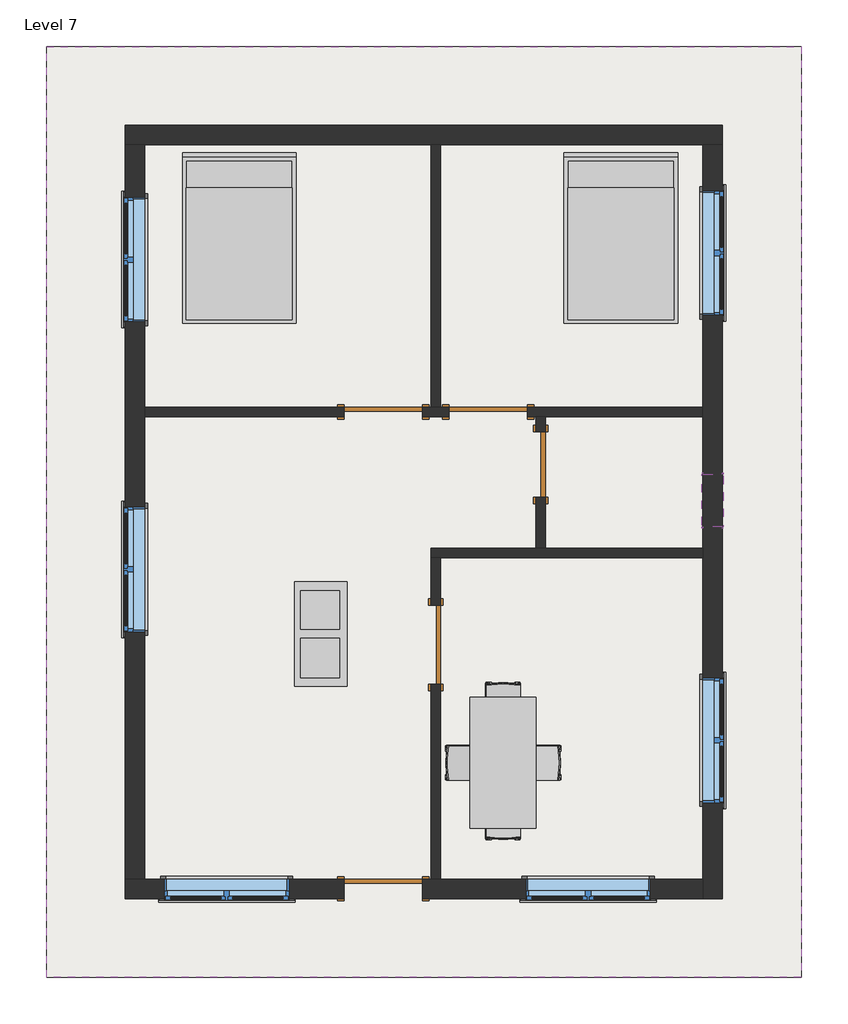
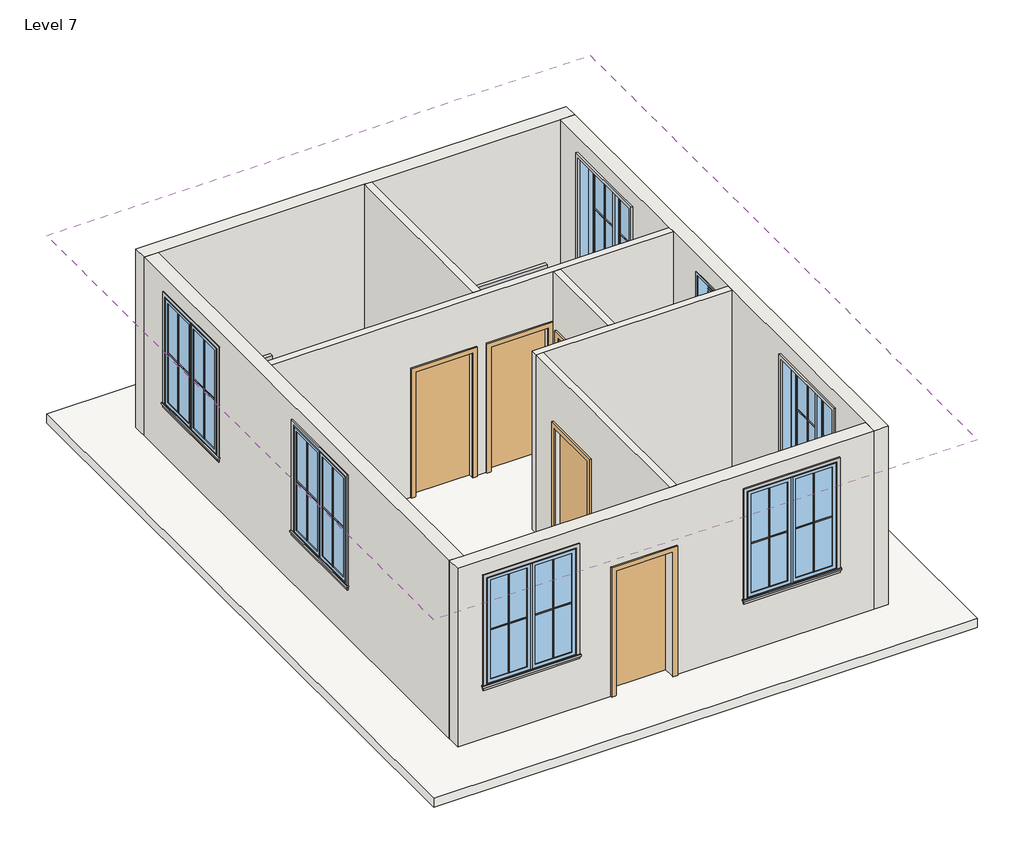
# One storey, incomplete: 25 proxies, 9 walls, 7 windows, 5 doors, 3 furniture elements, 2 roofs.
"""IFC4 building model written with IfcOpenShell, lengths in millimetres."""

from ifc_helpers import new_model, si_unit, frame, origin, place, context, project, spatial, polyline, outline, extrude, faceted_brep, transform, mapped, element, save
from components import muntin_pattern_2x2_muntin_pattern_2x2_bff912c5, muntin_pattern_2x2_muntin_pattern_2x2_c2194282, trim_window_exterior_flat_with_sill_e04b3088, trim_window_interior_flat_picture_frame_2a7685fe, coffee_table_with_brass_mullions_11320_coffee_table_with_5962bef7, door_305aa2a5, door_e5f9f3c4, door_0ca8825f, door_f2b275c1, bed_17739_bed_17739_15c61121, dining_table_w_chairs_11374_0cdfc61b, window_9ac97e1a, window_f2d8fef0

model = new_model("IFC4")

# Units and contexts
model_context = context("Model", 3, world=origin())
ifc_project = project(units=[si_unit("LENGTHUNIT", "METRE", prefix="MILLI")], contexts=[model_context])

# Site, building, storey
site = spatial("IfcSite", under=ifc_project)
building = spatial("IfcBuilding", under=site)
storey = spatial("IfcBuildingStorey", under=building, Name="Level 7", Elevation=19050.0)

# Proxies
placement = place(None, origin())
muntin_pattern_2x2_muntin_pattern_2x2_shape = muntin_pattern_2x2_muntin_pattern_2x2_bff912c5(model_context)
element("IfcBuildingElementProxy", 1, Name="Muntin Pattern_2x2 : Muntin Pattern_2x2", ObjectType="Muntin Pattern_2x2 : Muntin Pattern_2x2", at=placement, inside=storey, context=model_context, shape_type="MappedRepresentation", body=[
    mapped(muntin_pattern_2x2_muntin_pattern_2x2_shape, transform((-4718.1437352, -1580.3188735, 20034.25), x_axis=(0.0, 1.0, 0.0), y_axis=(-1.0, 0.0, 0.0), z_axis=(0.0, 0.0, 1.0))),
])
element("IfcBuildingElementProxy", 2, Name="Muntin Pattern_2x2 : Muntin Pattern_2x2", ObjectType="Muntin Pattern_2x2 : Muntin Pattern_2x2", at=placement, inside=storey, context=model_context, shape_type="MappedRepresentation", body=[
    mapped(muntin_pattern_2x2_muntin_pattern_2x2_shape, transform((-3186.2062352, -5039.4813735, 20034.25), x_axis=(-1.0, 0.0, 0.0), y_axis=(0.0, -1.0, 0.0), z_axis=(0.0, 0.0, 1.0))),
])
element("IfcBuildingElementProxy", 3, Name="Muntin Pattern_2x2 : Muntin Pattern_2x2", ObjectType="Muntin Pattern_2x2 : Muntin Pattern_2x2", at=placement, inside=storey, context=model_context, shape_type="MappedRepresentation", body=[
    mapped(muntin_pattern_2x2_muntin_pattern_2x2_shape, transform((1017.4937648, -5039.4813735, 20034.25), x_axis=(-1.0, 0.0, 0.0), y_axis=(0.0, -1.0, 0.0), z_axis=(0.0, 0.0, 1.0))),
])
element("IfcBuildingElementProxy", 4, Name="Muntin Pattern_2x2 : Muntin Pattern_2x2", ObjectType="Muntin Pattern_2x2 : Muntin Pattern_2x2", at=placement, inside=storey, context=model_context, shape_type="MappedRepresentation", body=[
    mapped(muntin_pattern_2x2_muntin_pattern_2x2_shape, transform((2209.7062648, -2847.1438735, 20034.25), x_axis=(0.0, -1.0, 0.0), y_axis=(1.0, 0.0, 0.0), z_axis=(0.0, 0.0, 1.0))),
])
element("IfcBuildingElementProxy", 5, Name="Muntin Pattern_2x2 : Muntin Pattern_2x2", ObjectType="Muntin Pattern_2x2 : Muntin Pattern_2x2", at=placement, inside=storey, context=model_context, shape_type="MappedRepresentation", body=[
    mapped(muntin_pattern_2x2_muntin_pattern_2x2_shape, transform((2209.7062648, 2817.0561265, 20034.25), x_axis=(0.0, -1.0, 0.0), y_axis=(1.0, 0.0, 0.0), z_axis=(0.0, 0.0, 1.0))),
])
element("IfcBuildingElementProxy", 6, Name="Muntin Pattern_2x2 : Muntin Pattern_2x2", ObjectType="Muntin Pattern_2x2 : Muntin Pattern_2x2", at=placement, inside=storey, context=model_context, shape_type="MappedRepresentation", body=[
    mapped(muntin_pattern_2x2_muntin_pattern_2x2_shape, transform((-4718.1437352, 2020.1311265, 20034.25), x_axis=(0.0, 1.0, 0.0), y_axis=(-1.0, 0.0, 0.0), z_axis=(0.0, 0.0, 1.0))),
])
muntin_pattern_2x2_muntin_pattern_2x2_2_shape = muntin_pattern_2x2_muntin_pattern_2x2_c2194282(model_context)
element("IfcBuildingElementProxy", 7, Name="Muntin Pattern_2x2 : Muntin Pattern_2x2", ObjectType="Muntin Pattern_2x2 : Muntin Pattern_2x2", at=placement, inside=storey, context=model_context, shape_type="MappedRepresentation", body=[
    mapped(muntin_pattern_2x2_muntin_pattern_2x2_2_shape, transform((-4718.1437352, -859.5938735, 20034.25), x_axis=(0.0, -1.0, 0.0), y_axis=(1.0, 0.0, 0.0), z_axis=(0.0, 0.0, 1.0))),
])
element("IfcBuildingElementProxy", 8, Name="Muntin Pattern_2x2 : Muntin Pattern_2x2", ObjectType="Muntin Pattern_2x2 : Muntin Pattern_2x2", at=placement, inside=storey, context=model_context, shape_type="MappedRepresentation", body=[
    mapped(muntin_pattern_2x2_muntin_pattern_2x2_2_shape, transform((-3906.9312352, -5039.4813735, 20034.25), x_axis=(1.0, 0.0, 0.0), y_axis=(0.0, 1.0, 0.0), z_axis=(0.0, 0.0, 1.0))),
])
element("IfcBuildingElementProxy", 9, Name="Muntin Pattern_2x2 : Muntin Pattern_2x2", ObjectType="Muntin Pattern_2x2 : Muntin Pattern_2x2", at=placement, inside=storey, context=model_context, shape_type="MappedRepresentation", body=[
    mapped(muntin_pattern_2x2_muntin_pattern_2x2_2_shape, transform((296.7687648, -5039.4813735, 20034.25), x_axis=(1.0, 0.0, 0.0), y_axis=(0.0, 1.0, 0.0), z_axis=(0.0, 0.0, 1.0))),
])
element("IfcBuildingElementProxy", 10, Name="Muntin Pattern_2x2 : Muntin Pattern_2x2", ObjectType="Muntin Pattern_2x2 : Muntin Pattern_2x2", at=placement, inside=storey, context=model_context, shape_type="MappedRepresentation", body=[
    mapped(muntin_pattern_2x2_muntin_pattern_2x2_2_shape, transform((2209.7062648, -3567.8688735, 20034.25), x_axis=(0.0, 1.0, 0.0), y_axis=(-1.0, 0.0, 0.0), z_axis=(0.0, 0.0, 1.0))),
])
element("IfcBuildingElementProxy", 11, Name="Muntin Pattern_2x2 : Muntin Pattern_2x2", ObjectType="Muntin Pattern_2x2 : Muntin Pattern_2x2", at=placement, inside=storey, context=model_context, shape_type="MappedRepresentation", body=[
    mapped(muntin_pattern_2x2_muntin_pattern_2x2_2_shape, transform((2209.7062648, 2096.3311265, 20034.25), x_axis=(0.0, 1.0, 0.0), y_axis=(-1.0, 0.0, 0.0), z_axis=(0.0, 0.0, 1.0))),
])
element("IfcBuildingElementProxy", 12, Name="Muntin Pattern_2x2 : Muntin Pattern_2x2", ObjectType="Muntin Pattern_2x2 : Muntin Pattern_2x2", at=placement, inside=storey, context=model_context, shape_type="MappedRepresentation", body=[
    mapped(muntin_pattern_2x2_muntin_pattern_2x2_2_shape, transform((-4718.1437352, 2740.8561265, 20034.25), x_axis=(0.0, -1.0, 0.0), y_axis=(1.0, 0.0, 0.0), z_axis=(0.0, 0.0, 1.0))),
])
trim_window_exterior_flat_with_sill_shape = trim_window_exterior_flat_with_sill_e04b3088(model_context)
element("IfcBuildingElementProxy", 13, Name="Trim-Window-Exterior-Flat : with Sill", ObjectType="Trim-Window-Exterior-Flat : with Sill", at=placement, inside=storey, context=model_context, shape_type="MappedRepresentation", body=[
    mapped(trim_window_exterior_flat_with_sill_shape, transform((-4727.6687352, -1219.9563735, 21793.2), x_axis=(0.0, -1.0, 0.0), y_axis=(0.0, 0.0, 1.0), z_axis=(-1.0, 0.0, 0.0))),
])
element("IfcBuildingElementProxy", 14, Name="Trim-Window-Exterior-Flat : with Sill", ObjectType="Trim-Window-Exterior-Flat : with Sill", at=placement, inside=storey, context=model_context, shape_type="MappedRepresentation", body=[
    mapped(trim_window_exterior_flat_with_sill_shape, transform((-3546.5687352, -5049.0063735, 21793.2), x_axis=(1.0, 0.0, 0.0), y_axis=(0.0, 0.0, 1.0), z_axis=(0.0, -1.0, 0.0))),
])
element("IfcBuildingElementProxy", 15, Name="Trim-Window-Exterior-Flat : with Sill", ObjectType="Trim-Window-Exterior-Flat : with Sill", at=placement, inside=storey, context=model_context, shape_type="MappedRepresentation", body=[
    mapped(trim_window_exterior_flat_with_sill_shape, transform((657.1312648, -5049.0063735, 21793.2), x_axis=(1.0, 0.0, 0.0), y_axis=(0.0, 0.0, 1.0), z_axis=(0.0, -1.0, 0.0))),
])
element("IfcBuildingElementProxy", 16, Name="Trim-Window-Exterior-Flat : with Sill", ObjectType="Trim-Window-Exterior-Flat : with Sill", at=placement, inside=storey, context=model_context, shape_type="MappedRepresentation", body=[
    mapped(trim_window_exterior_flat_with_sill_shape, transform((2219.2312648, -3207.5063735, 21793.2), x_axis=(0.0, 1.0, 0.0), y_axis=(0.0, 0.0, 1.0), z_axis=(1.0, 0.0, 0.0))),
])
element("IfcBuildingElementProxy", 17, Name="Trim-Window-Exterior-Flat : with Sill", ObjectType="Trim-Window-Exterior-Flat : with Sill", at=placement, inside=storey, context=model_context, shape_type="MappedRepresentation", body=[
    mapped(trim_window_exterior_flat_with_sill_shape, transform((2219.2312648, 2456.6936265, 21793.2), x_axis=(0.0, 1.0, 0.0), y_axis=(0.0, 0.0, 1.0), z_axis=(1.0, 0.0, 0.0))),
])
element("IfcBuildingElementProxy", 18, Name="Trim-Window-Exterior-Flat : with Sill", ObjectType="Trim-Window-Exterior-Flat : with Sill", at=placement, inside=storey, context=model_context, shape_type="MappedRepresentation", body=[
    mapped(trim_window_exterior_flat_with_sill_shape, transform((-4727.6687352, 2380.4936265, 21793.2), x_axis=(0.0, -1.0, 0.0), y_axis=(0.0, 0.0, 1.0), z_axis=(-1.0, 0.0, 0.0))),
])
trim_window_interior_flat_picture_frame_shape = trim_window_interior_flat_picture_frame_2a7685fe(model_context)
element("IfcBuildingElementProxy", 19, Name="Trim-Window-Interior-Flat : Picture Frame", ObjectType="Trim-Window-Interior-Flat : Picture Frame", at=placement, inside=storey, context=model_context, shape_type="MappedRepresentation", body=[
    mapped(trim_window_interior_flat_picture_frame_shape, transform((-4499.0687352, -1219.9563735, 21793.2), x_axis=(0.0, 1.0, 0.0), y_axis=(0.0, 0.0, 1.0), z_axis=(1.0, 0.0, 0.0))),
])
element("IfcBuildingElementProxy", 20, Name="Trim-Window-Interior-Flat : Picture Frame", ObjectType="Trim-Window-Interior-Flat : Picture Frame", at=placement, inside=storey, context=model_context, shape_type="MappedRepresentation", body=[
    mapped(trim_window_interior_flat_picture_frame_shape, transform((-3546.5687352, -4820.4063735, 21793.2), x_axis=(-1.0, 0.0, 0.0), y_axis=(0.0, 0.0, 1.0), z_axis=(0.0, 1.0, 0.0))),
])
element("IfcBuildingElementProxy", 21, Name="Trim-Window-Interior-Flat : Picture Frame", ObjectType="Trim-Window-Interior-Flat : Picture Frame", at=placement, inside=storey, context=model_context, shape_type="MappedRepresentation", body=[
    mapped(trim_window_interior_flat_picture_frame_shape, transform((657.1312648, -4820.4063735, 21793.2), x_axis=(-1.0, 0.0, 0.0), y_axis=(0.0, 0.0, 1.0), z_axis=(0.0, 1.0, 0.0))),
])
element("IfcBuildingElementProxy", 22, Name="Trim-Window-Interior-Flat : Picture Frame", ObjectType="Trim-Window-Interior-Flat : Picture Frame", at=placement, inside=storey, context=model_context, shape_type="MappedRepresentation", body=[
    mapped(trim_window_interior_flat_picture_frame_shape, transform((1990.6312648, -3207.5063735, 21793.2), x_axis=(0.0, -1.0, 0.0), y_axis=(0.0, 0.0, 1.0), z_axis=(-1.0, 0.0, 0.0))),
])
element("IfcBuildingElementProxy", 23, Name="Trim-Window-Interior-Flat : Picture Frame", ObjectType="Trim-Window-Interior-Flat : Picture Frame", at=placement, inside=storey, context=model_context, shape_type="MappedRepresentation", body=[
    mapped(trim_window_interior_flat_picture_frame_shape, transform((1990.6312648, 2456.6936265, 21793.2), x_axis=(0.0, -1.0, 0.0), y_axis=(0.0, 0.0, 1.0), z_axis=(-1.0, 0.0, 0.0))),
])
element("IfcBuildingElementProxy", 24, Name="Trim-Window-Interior-Flat : Picture Frame", ObjectType="Trim-Window-Interior-Flat : Picture Frame", at=placement, inside=storey, context=model_context, shape_type="MappedRepresentation", body=[
    mapped(trim_window_interior_flat_picture_frame_shape, transform((-4499.0687352, 2380.4936265, 21793.2), x_axis=(0.0, 1.0, 0.0), y_axis=(0.0, 0.0, 1.0), z_axis=(1.0, 0.0, 0.0))),
])
coffee_table_with_brass_mullions_11320_coffee_table_with_shape = coffee_table_with_brass_mullions_11320_coffee_table_with_5962bef7(model_context)
element("IfcBuildingElementProxy", 25, Name="coffee_table_with_brass_mullions_11320 : coffee_table_with_brass_mullions_11320", ObjectType="coffee_table_with_brass_mullions_11320 : coffee_table_with_brass_mullions_11320", at=placement, inside=storey, context=model_context, shape_type="MappedRepresentation", body=[
    mapped(coffee_table_with_brass_mullions_11320_coffee_table_with_shape, transform((-2022.5687352, -1334.2563735, 19050.0), x_axis=(0.0, 1.0, 0.0), y_axis=(-1.0, 0.0, 0.0), z_axis=(0.0, 0.0, 1.0))),
])

# Doors
door_shape = door_305aa2a5(model_context)
element("IfcDoor", 26, ObjectType="Single-Flush : 36\" x 84\"", at=placement, inside=storey, context=model_context, shape_type="MappedRepresentation", body=[
    mapped(door_shape, transform((-1114.5187352, -2096.2563735, 19050.0), x_axis=(0.0, 1.0, 0.0), y_axis=(-1.0, 0.0, 0.0), z_axis=(0.0, 0.0, 1.0))),
])
element("IfcDoor", 27, ObjectType="Single-Flush : 36\" x 84\"", at=placement, inside=storey, context=model_context, shape_type="MappedRepresentation", body=[
    mapped(door_shape, transform((-1724.1187352, 608.8436265, 19050.0), x_axis=(-1.0, 0.0, 0.0), y_axis=(0.0, -1.0, 0.0), z_axis=(0.0, 0.0, 1.0))),
])
door_2_shape = door_e5f9f3c4(model_context)
element("IfcDoor", 28, ObjectType="Single-Flush : 36\" x 84\"", at=placement, inside=storey, context=model_context, shape_type="MappedRepresentation", body=[
    mapped(door_2_shape, transform((-504.9187352, 608.8436265, 19050.0), x_axis=(1.0, 0.0, 0.0), y_axis=(0.0, 1.0, 0.0), z_axis=(0.0, 0.0, 1.0))),
])
door_3_shape = door_0ca8825f(model_context)
element("IfcDoor", 29, ObjectType="Single-Flush : 36\" x 84\"", at=placement, inside=storey, context=model_context, shape_type="MappedRepresentation", body=[
    mapped(door_3_shape, transform((-1724.1187352, -4934.7063735, 19050.0), x_axis=(1.0, 0.0, 0.0), y_axis=(0.0, 1.0, 0.0), z_axis=(0.0, 0.0, 1.0))),
])
door_4_shape = door_f2b275c1(model_context)
element("IfcDoor", 30, ObjectType="Single-Flush : DOOR 2'6\"", at=placement, inside=storey, context=model_context, shape_type="MappedRepresentation", body=[
    mapped(door_4_shape, transform((104.6812648, -0.7563735, 19050.0), x_axis=(0.0, 1.0, 0.0), y_axis=(-1.0, 0.0, 0.0), z_axis=(0.0, 0.0, 1.0))),
])

# Furniture
bed_17739_bed_17739_shape = bed_17739_bed_17739_15c61121(model_context)
element("IfcFurniture", 31, ObjectType="Bed_17739 : Bed_17739", at=placement, inside=storey, context=model_context, shape_type="MappedRepresentation", body=[
    mapped(bed_17739_bed_17739_shape, transform((-3400.5187352, 2609.0936265, 19050.0), x_axis=(1.0, 0.0, 0.0), y_axis=(0.0, 1.0, 0.0), z_axis=(0.0, 0.0, 1.0))),
])
element("IfcFurniture", 32, ObjectType="Bed_17739 : Bed_17739", at=placement, inside=storey, context=model_context, shape_type="MappedRepresentation", body=[
    mapped(bed_17739_bed_17739_shape, transform((1038.1312648, 2609.0936265, 19050.0), x_axis=(1.0, 0.0, 0.0), y_axis=(0.0, 1.0, 0.0), z_axis=(0.0, 0.0, 1.0))),
])
dining_table_w_chairs_11374_shape = dining_table_w_chairs_11374_0cdfc61b(model_context)
element("IfcFurniture", 33, ObjectType="Dining_Table_w_Chairs_11374", at=placement, inside=storey, context=model_context, shape_type="MappedRepresentation", body=[
    mapped(dining_table_w_chairs_11374_shape, transform((-238.2576574, -3486.1221401, 19050.0), x_axis=(0.0, 1.0, 0.0), y_axis=(-1.0, 0.0, 0.0), z_axis=(0.0, 0.0, 1.0))),
])

# Roofs
element("IfcRoof", 34, ObjectType="ROOF 6\"", at=placement, inside=storey, context=model_context, shape_type="SweptSolid", body=[
    extrude(outline(polyline([(-5642.0687352, 4856.9936265), (3133.6312648, 4856.9936265), (3133.6312648, -5963.4063735), (-5642.0687352, -5963.4063735), (-5642.0687352, 4856.9936265)])), frame((0.0, 0.0, 18897.6), z_axis=(0.0, 0.0, 1.0), x_axis=(1.0, 0.0, 0.0)), (0.0, 0.0, 1.0), 152.4),
])
element("IfcRoof", 35, ObjectType="ROOF 6\"", at=placement, inside=storey, context=model_context, shape_type="SweptSolid", body=[
    extrude(outline(polyline([(-5642.0687352, 4856.9936265), (3133.6312648, 4856.9936265), (3133.6312648, -5963.4063735), (-5642.0687352, -5963.4063735), (-5642.0687352, 4856.9936265)])), frame((0.0, 0.0, 22098.0), z_axis=(0.0, 0.0, 1.0), x_axis=(1.0, 0.0, 0.0)), (0.0, 0.0, 1.0), 152.4),
])

# Walls
element("IfcWall", 36, ObjectType="WALL 4.5\"", at=placement, inside=storey, context=model_context, shape_type="Brep", body=[
    faceted_brep([(-4499.0687352, 551.6936265, 19050.0), (-2181.3187352, 551.6936265, 19050.0), (-2181.3187352, 551.6936265, 21183.6), (-1266.9187352, 551.6936265, 21183.6), (-1266.9187352, 551.6936265, 19050.0), (-962.1187352, 551.6936265, 19050.0), (-962.1187352, 551.6936265, 21183.6), (-47.7187352, 551.6936265, 21183.6), (-47.7187352, 551.6936265, 19050.0), (47.5312648, 551.6936265, 19050.0), (161.8312648, 551.6936265, 19050.0), (1990.6312648, 551.6936265, 19050.0), (1990.6312648, 551.6936265, 22098.0), (161.8312648, 551.6936265, 22098.0), (47.5312648, 551.6936265, 22098.0), (-4499.0687352, 551.6936265, 22098.0), (-2181.3187352, 665.9936265, 21183.6), (-2181.3187352, 665.9936265, 19050.0), (-4499.0687352, 665.9936265, 19050.0), (-4499.0687352, 665.9936265, 22098.0), (-1171.6687352, 665.9936265, 22098.0), (-1057.3687352, 665.9936265, 22098.0), (1990.6312648, 665.9936265, 22098.0), (1990.6312648, 665.9936265, 19050.0), (-47.7187352, 665.9936265, 19050.0), (-47.7187352, 665.9936265, 21183.6), (-962.1187352, 665.9936265, 21183.6), (-962.1187352, 665.9936265, 19050.0), (-1057.3687352, 665.9936265, 19050.0), (-1171.6687352, 665.9936265, 19050.0), (-1266.9187352, 665.9936265, 19050.0), (-1266.9187352, 665.9936265, 21183.6)], [[[0, 1, 2, 3, 4, 5, 6, 7, 8, 9, 10, 11, 12, 13, 14, 15]], [[16, 17, 18, 19, 20, 21, 22, 23, 24, 25, 26, 27, 28, 29, 30, 31]], [[11, 10, 9, 8, 24, 23]], [[18, 17, 1, 0]], [[30, 29, 28, 27, 5, 4]], [[12, 11, 23, 22]], [[0, 15, 19, 18]], [[25, 24, 8, 7]], [[26, 25, 7, 6]], [[27, 26, 6, 5]], [[2, 1, 17, 16]], [[3, 2, 16, 31]], [[4, 3, 31, 30]], [[15, 14, 13, 12, 22, 21, 20, 19]]]),
])
element("IfcWall", 37, ObjectType="WALL 4.5\"", at=placement, inside=storey, context=model_context, shape_type="SweptSolid", body=[
    extrude(outline(polyline([(-1057.3687352, 3713.9936265), (-1057.3687352, 665.9936265), (-1171.6687352, 665.9936265), (-1171.6687352, 3713.9936265), (-1057.3687352, 3713.9936265)])), frame((0.0, 0.0, 19050.0), z_axis=(0.0, 0.0, 1.0), x_axis=(1.0, 0.0, 0.0)), (0.0, 0.0, 1.0), 3048.0),
])
element("IfcWall", 38, ObjectType="WALL 4.5\"", at=placement, inside=storey, context=model_context, shape_type="Brep", body=[
    faceted_brep([(1990.6312648, -972.3063735, 19050.0), (161.8312648, -972.3063735, 19050.0), (47.5312648, -972.3063735, 19050.0), (-1171.6687352, -972.3063735, 19050.0), (-1171.6687352, -972.3063735, 22098.0), (47.5312648, -972.3063735, 22098.0), (161.8312648, -972.3063735, 22098.0), (1990.6312648, -972.3063735, 22098.0), (1990.6312648, -1086.6063735, 19050.0), (1990.6312648, -1086.6063735, 22098.0), (-1057.3687352, -1086.6063735, 22098.0), (-1171.6687352, -1086.6063735, 22098.0), (-1171.6687352, -1086.6063735, 19050.0), (-1057.3687352, -1086.6063735, 19050.0)], [[[0, 1, 2, 3, 4, 5, 6, 7]], [[8, 9, 10, 11, 12, 13]], [[3, 2, 1, 0, 8, 13, 12]], [[0, 7, 9, 8]], [[4, 3, 12, 11]], [[7, 6, 5, 4, 11, 10, 9]]]),
])
element("IfcWall", 39, ObjectType="WALL 4.5\"", at=placement, inside=storey, context=model_context, shape_type="SweptSolid", body=[
    extrude(outline(polyline([(-1086.6063735, 19050.0), (-1639.0563735, 19050.0), (-1639.0563735, 21183.6), (-2553.4563735, 21183.6), (-2553.4563735, 19050.0), (-4820.4063735, 19050.0), (-4820.4063735, 22098.0), (-1086.6063735, 22098.0), (-1086.6063735, 19050.0)])), frame((-1171.6687352, 0.0, 0.0), z_axis=(1.0, 0.0, 0.0), x_axis=(0.0, 1.0, 0.0)), (0.0, 0.0, 1.0), 114.3),
])
element("IfcWall", 40, ObjectType="WALL 4.5\"", at=placement, inside=storey, context=model_context, shape_type="SweptSolid", body=[
    extrude(outline(polyline([(551.6936265, 19050.0), (380.2436265, 19050.0), (380.2436265, 21082.0), (-381.7563735, 21082.0), (-381.7563735, 19050.0), (-972.3063735, 19050.0), (-972.3063735, 22098.0), (551.6936265, 22098.0), (551.6936265, 19050.0)])), frame((47.5312648, 0.0, 0.0), z_axis=(1.0, 0.0, 0.0), x_axis=(0.0, 1.0, 0.0)), (0.0, 0.0, 1.0), 114.3),
])
element("IfcWall", 41, ObjectType="WALL 9\"", at=placement, inside=storey, context=model_context, shape_type="Brep", body=[
    faceted_brep([(-4727.6687352, 3713.9936265, 19050.0), (-4499.0687352, 3713.9936265, 19050.0), (-1171.6687352, 3713.9936265, 19050.0), (-1057.3687352, 3713.9936265, 19050.0), (1990.6312648, 3713.9936265, 19050.0), (2219.2312648, 3713.9936265, 19050.0), (2219.2312648, 3713.9936265, 22098.0), (1990.6312648, 3713.9936265, 22098.0), (-1057.3687352, 3713.9936265, 22098.0), (-1171.6687352, 3713.9936265, 22098.0), (-4499.0687352, 3713.9936265, 22098.0), (-4727.6687352, 3713.9936265, 22098.0), (-4727.6687352, 3942.5936265, 19050.0), (-4727.6687352, 3942.5936265, 22098.0), (2219.2312648, 3942.5936265, 22098.0), (2219.2312648, 3942.5936265, 19050.0)], [[[0, 1, 2, 3, 4, 5, 6, 7, 8, 9, 10, 11]], [[12, 13, 14, 15]], [[5, 4, 3, 2, 1, 0, 12, 15]], [[6, 5, 15, 14]], [[0, 11, 13, 12]], [[11, 10, 9, 8, 7, 6, 14, 13]]]),
])
element("IfcWall", 42, ObjectType="WALL 9\"", at=placement, inside=storey, context=model_context, shape_type="Brep", body=[
    faceted_brep([(1990.6312648, 3713.9936265, 19050.0), (1990.6312648, 665.9936265, 19050.0), (1990.6312648, 551.6936265, 19050.0), (1990.6312648, -972.3063735, 19050.0), (1990.6312648, -1086.6063735, 19050.0), (1990.6312648, -4820.4063735, 19050.0), (1990.6312648, -5049.0063735, 19050.0), (1990.6312648, -5049.0063735, 22098.0), (1990.6312648, -4820.4063735, 22098.0), (1990.6312648, -1086.6063735, 22098.0), (1990.6312648, -972.3063735, 22098.0), (1990.6312648, 551.6936265, 22098.0), (1990.6312648, 665.9936265, 22098.0), (1990.6312648, 3713.9936265, 22098.0), (1990.6312648, -3931.4063735, 21793.2), (1990.6312648, -3931.4063735, 19964.4), (1990.6312648, -2483.6063735, 19964.4), (1990.6312648, -2483.6063735, 21793.2), (1990.6312648, 1732.7936265, 21793.2), (1990.6312648, 1732.7936265, 19964.4), (1990.6312648, 3180.5936265, 19964.4), (1990.6312648, 3180.5936265, 21793.2), (1990.6312648, -115.0563735, 21793.2), (1990.6312648, -724.6563735, 21793.2), (1990.6312648, -724.6563735, 21183.6), (1990.6312648, -115.0563735, 21183.6), (2219.2312648, 3713.9936265, 19050.0), (2219.2312648, 3713.9936265, 22098.0), (2219.2312648, -5049.0063735, 22098.0), (2219.2312648, -5049.0063735, 19050.0), (2219.2312648, -3931.4063735, 21793.2), (2219.2312648, -2483.6063735, 21793.2), (2219.2312648, -2483.6063735, 19964.4), (2219.2312648, -3931.4063735, 19964.4), (2219.2312648, 1732.7936265, 21793.2), (2219.2312648, 3180.5936265, 21793.2), (2219.2312648, 3180.5936265, 19964.4), (2219.2312648, 1732.7936265, 19964.4), (2219.2312648, -115.0563735, 21793.2), (2219.2312648, -115.0563735, 21183.6), (2219.2312648, -724.6563735, 21183.6), (2219.2312648, -724.6563735, 21793.2)], [[[0, 1, 2, 3, 4, 5, 6, 7, 8, 9, 10, 11, 12, 13], [14, 15, 16, 17], [18, 19, 20, 21], [22, 23, 24, 25]], [[26, 27, 28, 29], [30, 31, 32, 33], [34, 35, 36, 37], [38, 39, 40, 41]], [[6, 5, 4, 3, 2, 1, 0, 26, 29]], [[0, 13, 27, 26]], [[7, 6, 29, 28]], [[15, 14, 30, 33]], [[16, 15, 33, 32]], [[17, 16, 32, 31]], [[14, 17, 31, 30]], [[19, 18, 34, 37]], [[20, 19, 37, 36]], [[21, 20, 36, 35]], [[18, 21, 35, 34]], [[39, 38, 22, 25]], [[40, 39, 25, 24]], [[41, 40, 24, 23]], [[38, 41, 23, 22]], [[13, 12, 11, 10, 9, 8, 7, 28, 27]]]),
])
element("IfcWall", 43, ObjectType="WALL 9\"", at=placement, inside=storey, context=model_context, shape_type="Brep", body=[
    faceted_brep([(1990.6312648, -4820.4063735, 19050.0), (-1057.3687352, -4820.4063735, 19050.0), (-1171.6687352, -4820.4063735, 19050.0), (-1266.9187352, -4820.4063735, 19050.0), (-1266.9187352, -4820.4063735, 21183.6), (-2181.3187352, -4820.4063735, 21183.6), (-2181.3187352, -4820.4063735, 19050.0), (-4499.0687352, -4820.4063735, 19050.0), (-4727.6687352, -4820.4063735, 19050.0), (-4727.6687352, -4820.4063735, 22098.0), (-4499.0687352, -4820.4063735, 22098.0), (-1171.6687352, -4820.4063735, 22098.0), (-1057.3687352, -4820.4063735, 22098.0), (1990.6312648, -4820.4063735, 22098.0), (-4270.4687352, -4820.4063735, 21793.2), (-4270.4687352, -4820.4063735, 19964.4), (-2822.6687352, -4820.4063735, 19964.4), (-2822.6687352, -4820.4063735, 21793.2), (-66.7687352, -4820.4063735, 21793.2), (-66.7687352, -4820.4063735, 19964.4), (1381.0312648, -4820.4063735, 19964.4), (1381.0312648, -4820.4063735, 21793.2), (-1266.9187352, -5049.0063735, 21183.6), (-1266.9187352, -5049.0063735, 19050.0), (1990.6312648, -5049.0063735, 19050.0), (1990.6312648, -5049.0063735, 22098.0), (-4727.6687352, -5049.0063735, 22098.0), (-4727.6687352, -5049.0063735, 19050.0), (-2181.3187352, -5049.0063735, 19050.0), (-2181.3187352, -5049.0063735, 21183.6), (-4270.4687352, -5049.0063735, 21793.2), (-2822.6687352, -5049.0063735, 21793.2), (-2822.6687352, -5049.0063735, 19964.4), (-4270.4687352, -5049.0063735, 19964.4), (-66.7687352, -5049.0063735, 21793.2), (1381.0312648, -5049.0063735, 21793.2), (1381.0312648, -5049.0063735, 19964.4), (-66.7687352, -5049.0063735, 19964.4)], [[[0, 1, 2, 3, 4, 5, 6, 7, 8, 9, 10, 11, 12, 13], [14, 15, 16, 17], [18, 19, 20, 21]], [[22, 23, 24, 25, 26, 27, 28, 29], [30, 31, 32, 33], [34, 35, 36, 37]], [[28, 27, 8, 7, 6]], [[24, 23, 3, 2, 1, 0]], [[0, 13, 25, 24]], [[9, 8, 27, 26]], [[15, 14, 30, 33]], [[16, 15, 33, 32]], [[17, 16, 32, 31]], [[14, 17, 31, 30]], [[19, 18, 34, 37]], [[20, 19, 37, 36]], [[21, 20, 36, 35]], [[18, 21, 35, 34]], [[4, 3, 23, 22]], [[5, 4, 22, 29]], [[6, 5, 29, 28]], [[13, 12, 11, 10, 9, 26, 25]]]),
])
element("IfcWall", 44, ObjectType="WALL 9\"", at=placement, inside=storey, context=model_context, shape_type="Brep", body=[
    faceted_brep([(-4499.0687352, -4820.4063735, 19050.0), (-4499.0687352, 551.6936265, 19050.0), (-4499.0687352, 665.9936265, 19050.0), (-4499.0687352, 3713.9936265, 19050.0), (-4499.0687352, 3713.9936265, 22098.0), (-4499.0687352, 665.9936265, 22098.0), (-4499.0687352, 551.6936265, 22098.0), (-4499.0687352, -4820.4063735, 22098.0), (-4499.0687352, -496.0563735, 21793.2), (-4499.0687352, -496.0563735, 19964.4), (-4499.0687352, -1943.8563735, 19964.4), (-4499.0687352, -1943.8563735, 21793.2), (-4499.0687352, 3104.3936265, 21793.2), (-4499.0687352, 3104.3936265, 19964.4), (-4499.0687352, 1656.5936265, 19964.4), (-4499.0687352, 1656.5936265, 21793.2), (-4727.6687352, -4820.4063735, 19050.0), (-4727.6687352, -4820.4063735, 22098.0), (-4727.6687352, 3713.9936265, 22098.0), (-4727.6687352, 3713.9936265, 19050.0), (-4727.6687352, -496.0563735, 21793.2), (-4727.6687352, -1943.8563735, 21793.2), (-4727.6687352, -1943.8563735, 19964.4), (-4727.6687352, -496.0563735, 19964.4), (-4727.6687352, 3104.3936265, 21793.2), (-4727.6687352, 1656.5936265, 21793.2), (-4727.6687352, 1656.5936265, 19964.4), (-4727.6687352, 3104.3936265, 19964.4)], [[[0, 1, 2, 3, 4, 5, 6, 7], [8, 9, 10, 11], [12, 13, 14, 15]], [[16, 17, 18, 19], [20, 21, 22, 23], [24, 25, 26, 27]], [[3, 2, 1, 0, 16, 19]], [[4, 3, 19, 18]], [[0, 7, 17, 16]], [[9, 8, 20, 23]], [[10, 9, 23, 22]], [[11, 10, 22, 21]], [[8, 11, 21, 20]], [[13, 12, 24, 27]], [[14, 13, 27, 26]], [[15, 14, 26, 25]], [[12, 15, 25, 24]], [[7, 6, 5, 4, 18, 17]]]),
])

# Windows
window_shape = window_9ac97e1a(model_context)
element("IfcWindow", 45, ObjectType="Window-Casement-Double : 57\" x 72\"", at=placement, inside=storey, context=model_context, shape_type="MappedRepresentation", body=[
    mapped(window_shape, transform((-4613.3687352, -1219.9563735, 19050.0), x_axis=(0.0, 1.0, 0.0), y_axis=(-1.0, 0.0, 0.0), z_axis=(0.0, 0.0, 1.0))),
])
element("IfcWindow", 46, ObjectType="Window-Casement-Double : 57\" x 72\"", at=placement, inside=storey, context=model_context, shape_type="MappedRepresentation", body=[
    mapped(window_shape, transform((-3546.5687352, -4934.7063735, 19050.0), x_axis=(-1.0, 0.0, 0.0), y_axis=(0.0, -1.0, 0.0), z_axis=(0.0, 0.0, 1.0))),
])
element("IfcWindow", 47, ObjectType="Window-Casement-Double : 57\" x 72\"", at=placement, inside=storey, context=model_context, shape_type="MappedRepresentation", body=[
    mapped(window_shape, transform((657.1312648, -4934.7063735, 19050.0), x_axis=(-1.0, 0.0, 0.0), y_axis=(0.0, -1.0, 0.0), z_axis=(0.0, 0.0, 1.0))),
])
element("IfcWindow", 48, ObjectType="Window-Casement-Double : 57\" x 72\"", at=placement, inside=storey, context=model_context, shape_type="MappedRepresentation", body=[
    mapped(window_shape, transform((2104.9312648, -3207.5063735, 19050.0), x_axis=(0.0, -1.0, 0.0), y_axis=(1.0, 0.0, 0.0), z_axis=(0.0, 0.0, 1.0))),
])
element("IfcWindow", 49, ObjectType="Window-Casement-Double : 57\" x 72\"", at=placement, inside=storey, context=model_context, shape_type="MappedRepresentation", body=[
    mapped(window_shape, transform((2104.9312648, 2456.6936265, 19050.0), x_axis=(0.0, -1.0, 0.0), y_axis=(1.0, 0.0, 0.0), z_axis=(0.0, 0.0, 1.0))),
])
element("IfcWindow", 50, ObjectType="Window-Casement-Double : 57\" x 72\"", at=placement, inside=storey, context=model_context, shape_type="MappedRepresentation", body=[
    mapped(window_shape, transform((-4613.3687352, 2380.4936265, 19050.0), x_axis=(0.0, 1.0, 0.0), y_axis=(-1.0, 0.0, 0.0), z_axis=(0.0, 0.0, 1.0))),
])
window_2_shape = window_f2d8fef0(model_context)
element("IfcWindow", 51, ObjectType="Window-Louvers : 24\" x 24\"", at=placement, inside=storey, context=model_context, shape_type="MappedRepresentation", body=[
    mapped(window_2_shape, transform((2111.2812648, -419.8563735, 20269.2), x_axis=(0.0, -1.0, 0.0), y_axis=(1.0, 0.0, 0.0), z_axis=(0.0, 0.0, 1.0))),
])

save(model, "model.ifc")

# Revit data of these elements
# Type "Muntin Pattern_2x2 : Muntin Pattern_2x2"
#   Width [instance default] = 4' - 0"
#   Thickness = 0' - 0 1/2"
#   Height [instance default] = 4' - 0"
#   Distance = 0' - 0 3/4"
#   Interior Material [instance default] = none
#   Exterior Material [instance default] = none
#   Default Elevation = 0
# Type "Trim-Window-Exterior-Flat : with Sill"
#   Trim Width = 0' - 2 1/4"
#   Trim Thickness_Picture Frame = 0' - 1 1/4"
#   Trim Thickness_with Sill = 0' - 0 3/4"
#   Sill Thickness = 0' - 1 1/4"
#   Opening Width [instance default] = 2' - 0"
#   Opening Height [instance default] = 3' - 0"
#   Default Elevation = 4' - 0"
#   Sill = yes
#   Picture Frame = no
#   Trim Material [instance default] = none
# Type "Trim-Window-Interior-Flat : Picture Frame"
#   Trim Thickness_Picture Frame = 0' - 1 1/4"
#   Trim Width = 0' - 2 1/4"
#   Trim Thickness_with Sill = 0' - 0 3/4"
#   Sill Thickness = 0' - 1 1/4"
#   Opening Width [instance default] = 2' - 0"
#   Opening Height [instance default] = 3' - 0"
#   Default Elevation = 4' - 0"
#   Sill = no
#   Picture Frame = yes
#   Trim Material [instance default] = none
# Type "coffee_table_with_brass_mullions_11320 : coffee_table_with_brass_mullions_11320"
#   Default Elevation = 0
# Type "Single-Flush : 36\" x 84\""
#   Type Mark = "1"
#   Construction Type Id = "MDOOR"
#   Assembly Code = "C1020"
#   Analytic Construction = "Metal"
#   Thickness = 0' - 2"
#   Heat Transfer Coefficient (U) = 0.651978 BTU/(h·ft²·°F)
#   Height = 7' - 0"
#   Trim Projection Ext = 0' - 1"
#   Trim Projection Int = 0' - 1"
#   Trim Width = 0' - 3"
#   Width = 3' - 0"
#   Define Thermal Properties by = 1
#   Define Thermal Properties by = 1
#   Door Material = Door - Panel
#   Frame Material = Door - Frame
#   Visual Light Transmittance = 0
#   Solar Heat Gain Coefficient = 0
#   Function = (empty or 0)
#   Wall Closure = (empty or 0)
# Type "Single-Flush : DOOR 2'6\""
#   Type Mark = "8"
#   Construction Type Id = "MDOOR"
#   Assembly Code = "C1020"
#   Analytic Construction = "Metal"
#   Thickness = 0' - 2"
#   Heat Transfer Coefficient (U) = 0.651978 BTU/(h·ft²·°F)
#   Height = 6' - 8"
#   Trim Projection Ext = 0' - 1"
#   Trim Projection Int = 0' - 1"
#   Trim Width = 0' - 3"
#   Width = 2' - 6"
#   Define Thermal Properties by = 1
#   Door Material = Door - Panel
#   Frame Material = Door - Frame
#   Visual Light Transmittance = 0
#   Solar Heat Gain Coefficient = 0
#   Function = (empty or 0)
#   Wall Closure = (empty or 0)
# Type "Bed_17739 : Bed_17739"
#   Default Elevation = 0
# Type "Dining_Table_w_Chairs_11374"
#   Default Elevation = 0
#   Assembly Code = ""
# Type "ROOF 6\""
#   Assembly Code = "B1020"
#   Layers, outside or top first: 0' - 6" no material (function 1)
# Type "WALL 4.5\""
#   Assembly Code = "B2010"
#   Layers, outside or top first: 0' - 4 1/2" no material (function 1)
# Type "WALL 9\""
#   Assembly Code = "B2010"
#   Layers, outside or top first: 0' - 9" no material (function 1)
# Type "Window-Casement-Double : 57\" x 72\""
#   Type Mark = "17"
#   Fire Rating = "0.5h"
#   Assembly Code = "B2020100"
#   Analytic Construction = "Double glazing - domestic"
#   Frame Extension [instance default] = 0' - 0 1/4"
#   Window Inset [instance default] = 0' - 0"
#   Wall Thickness [instance default] = 0' - 6"
#   Interior Wall Closure [instance default] = 0' - 2 1/4"
#   Half Width = 2' - 4 1/2"
#   Visual Light Transmittance = 0.81
#   Thermal Resistance (R) = 1.8146 (h·ft²·°F)/BTU
#   Solar Heat Gain Coefficient = 0.76
#   Rough Width = 4' - 9 1/2"
#   Rough Height = 6' - 0 1/2"
#   Height = 6' - 0"
#   Heat Transfer Coefficient (U) = 0.5511 BTU/(h·ft²·°F)
#   Exterior Wall Closure [instance default] = 0' - 1 1/4"
#   Extension Jamb [instance default] = 0' - 2 1/4"
#   Default Sill Height = 3' - 0"
#   Width = 4' - 9"
#   Define Thermal Properties by = 0
#   Muntin Visibility = yes
#   Interior Trim Visibility [instance default] = yes
#   Exterior Trim Visibility [instance default] = yes
#   Extension Jamb Visibility [instance default] = yes
#   Interior Trim Material = Wood - Stained
#   Muntin Pattern = Muntin Pattern_2x2 : Muntin Pattern_2x2
#   Interior Trim = Trim-Window-Interior-Flat : Picture Frame
#   Interior Frame Material = Wood - Stained
#   Glass Panel Material = Glass
#   Exterior Trim Material = Clad - White
#   Exterior Trim = Trim-Window-Exterior-Flat : with Sill
#   Exterior Frame Material = Clad - White
#   Wall Closure = (empty or 0)
# Type "Window-Louvers : 24\" x 24\""
#   Type Mark = "18"
#   Construction Type Id = "GSP4R"
#   Assembly Code = "B20"
#   Analytic Construction = "1/8 in Pilkington single glazing"
#   Visual Light Transmittance = 0.9
#   Thermal Resistance (R) = 1.53941 (h·ft²·°F)/BTU
#   Solar Heat Gain Coefficient = 0.78
#   Max Height = 1' - 11.74264"
#   Height = 2' - 0"
#   Heat Transfer Coefficient (U) = 0.6496 BTU/(h·ft²·°F)
#   Blade Width [instance default] = 1' - 10 1/2"
#   Blade Vertical Thickness = 0' - 0.35355"
#   Blade Thickness = 0' - 0 1/4"
#   Blade Spacing = 0' - 1 1/2"
#   Blade Height = 0' - 1.85355"
#   Blade Depth = 0' - 3"
#   Blade Angle = 45.00°
#   Default Sill Height = 3' - 0"
#   Trim Projection_Exterior = 0' - 0 1/2"
#   Trim Projection_Interior = 0' - 0 1/2"
#   Trim Width_Exterior = 0' - 1 1/2"
#   Trim Width_Interior = 0' - 1 1/2"
#   Width = 2' - 0"
#   Max Blade Count = 12
#   Define Thermal Properties by = 1
#   Blade Count = 12
#   Frame Material = Birch
#   Louver Material = Birch
#   Trim Exterior Material = Birch
#   Trim Interior Material = Birch
#   Wall Closure = (empty or 0)
# Elements 1, 2, 3, 4, 5, 6, 7, 8, 9, 10, 11, 12 (IfcBuildingElementProxy, "Muntin Pattern_2x2 : Muntin Pattern_2x2")
#   Width = 1' - 11 1/8"
#   Height = 5' - 6 1/2"
#   Interior Material = Wood - Stained
#   Exterior Material = Clad - White
#   Phase Created = New Construction
#   Materials on its faces: "Clad - White", "Wood - Stained"
# Elements 13, 14, 15, 16, 17, 18 (IfcBuildingElementProxy, "Trim-Window-Exterior-Flat : with Sill")
#   Opening Width = 4' - 9"
#   Opening Height = 6' - 0"
#   Trim Material = Clad - White
#   Phase Created = New Construction
#   Materials on its faces: "Clad - White"
# Elements 19, 20, 21, 22, 23, 24 (IfcBuildingElementProxy, "Trim-Window-Interior-Flat : Picture Frame")
#   Opening Width = 4' - 9"
#   Opening Height = 6' - 0"
#   Trim Material = Wood - Stained
#   Phase Created = New Construction
#   Materials on its faces: "Wood - Stained"
# Element 25 (IfcBuildingElementProxy, "coffee_table_with_brass_mullions_11320 : coffee_table_with_brass_mullions_11320")
#   Phase Created = New Construction
#   Materials on its faces: "Default Wall", "TABLE", "Glass", "Default"
# Elements 26, 27, 28, 29 (IfcDoor, "Single-Flush : 36\" x 84\"")
#   Phase Created = New Construction
#   Materials on its faces: "Door - Frame", "Door - Panel"
# Element 30 (IfcDoor, "Single-Flush : DOOR 2'6\"")
#   Phase Created = New Construction
#   Materials on its faces: "Door - Frame", "Door - Panel"
# Elements 31, 32 (IfcFurniture, "Bed_17739 : Bed_17739")
#   Phase Created = New Construction
#   Materials on its faces: "legs", "sheets", "bed frame", "Blanket"
# Element 33 (IfcFurniture, "Dining_Table_w_Chairs_11374")
#   Phase Created = New Construction
# Element 34 (IfcRoof, "ROOF 6\"")
#   built-in parameter 1001705 = 62.5 (stored number, unit not read)
#   built-in parameter 1001701 = -0.5 (stored number, unit not read)
#   built-in parameter 1001710 = 33615
#   Phase Created = New Construction
#   Materials on its faces: "Copper", "Default Roof", "Wood - Stained"
# Element 35 (IfcRoof, "ROOF 6\"")
#   built-in parameter 1001705 = 73 (stored number, unit not read)
#   built-in parameter 1001701 = 10 (stored number, unit not read)
#   built-in parameter 1001710 = 33615
#   Phase Created = New Construction
#   Materials on its faces: "Copper", "Default Roof", "Wood - Stained"
# Elements 36, 37, 38, 39, 40 (IfcWall, "WALL 4.5\"")
#   Top Offset = 0' - 0"
#   Base Offset = 0' - 0"
#   Unconnected Height = 10' - 0"
#   wall height = 10' - 0"
#   Phase Created = New Construction
#   Base Constraint = Level 7
#   Materials on its faces: "Default Wall"
# Elements 41, 42, 43, 44 (IfcWall, "WALL 9\"")
#   Top Offset = 0' - 0"
#   Base Offset = 0' - 0"
#   Unconnected Height = 10' - 0"
#   wall height = 10' - 0"
#   Phase Created = New Construction
#   Base Constraint = Level 7
#   Materials on its faces: "Default Wall", "Parking Stripe"
# Element 45 (IfcWindow, "Window-Casement-Double : 57\" x 72\"")
#   Mark = "43"
#   Window Inset = 0' - 0"
#   Interior Wall Closure = 0' - 2 1/4"
#   Frame Extension = 0' - 0 1/4"
#   Exterior Wall Closure = 0' - 1 1/4"
#   Interior Trim Visibility = yes
#   Exterior Trim Visibility = yes
#   Phase Created = New Construction
#   Materials on its faces: "Wood - Stained", "Glass", "Clad - White"
# Element 46 (IfcWindow, "Window-Casement-Double : 57\" x 72\"")
#   Mark = "44"
#   Window Inset = 0' - 0"
#   Interior Wall Closure = 0' - 2 1/4"
#   Frame Extension = 0' - 0 1/4"
#   Exterior Wall Closure = 0' - 1 1/4"
#   Interior Trim Visibility = yes
#   Exterior Trim Visibility = yes
#   Phase Created = New Construction
#   Materials on its faces: "Wood - Stained", "Glass", "Clad - White"
# Element 47 (IfcWindow, "Window-Casement-Double : 57\" x 72\"")
#   Mark = "45"
#   Window Inset = 0' - 0"
#   Interior Wall Closure = 0' - 2 1/4"
#   Frame Extension = 0' - 0 1/4"
#   Exterior Wall Closure = 0' - 1 1/4"
#   Interior Trim Visibility = yes
#   Exterior Trim Visibility = yes
#   Phase Created = New Construction
#   Materials on its faces: "Wood - Stained", "Glass", "Clad - White"
# Element 48 (IfcWindow, "Window-Casement-Double : 57\" x 72\"")
#   Mark = "46"
#   Window Inset = 0' - 0"
#   Interior Wall Closure = 0' - 2 1/4"
#   Frame Extension = 0' - 0 1/4"
#   Exterior Wall Closure = 0' - 1 1/4"
#   Interior Trim Visibility = yes
#   Exterior Trim Visibility = yes
#   Phase Created = New Construction
#   Materials on its faces: "Wood - Stained", "Glass", "Clad - White"
# Element 49 (IfcWindow, "Window-Casement-Double : 57\" x 72\"")
#   Mark = "47"
#   Window Inset = 0' - 0"
#   Interior Wall Closure = 0' - 2 1/4"
#   Frame Extension = 0' - 0 1/4"
#   Exterior Wall Closure = 0' - 1 1/4"
#   Interior Trim Visibility = yes
#   Exterior Trim Visibility = yes
#   Phase Created = New Construction
#   Materials on its faces: "Wood - Stained", "Glass", "Clad - White"
# Element 50 (IfcWindow, "Window-Casement-Double : 57\" x 72\"")
#   Mark = "48"
#   Window Inset = 0' - 0"
#   Interior Wall Closure = 0' - 2 1/4"
#   Frame Extension = 0' - 0 1/4"
#   Exterior Wall Closure = 0' - 1 1/4"
#   Interior Trim Visibility = yes
#   Exterior Trim Visibility = yes
#   Phase Created = New Construction
#   Materials on its faces: "Wood - Stained", "Glass", "Clad - White"
# Element 51 (IfcWindow, "Window-Louvers : 24\" x 24\"")
#   Mark = "49"
#   Blade Width = 1' - 10 1/2"
#   Phase Created = New Construction
#   Materials on its faces: "Birch"
# Materials
#   "Door - Panel": class "Wood", colour RGB 210 159 95, transparency 0, Cost = 0
#   "Door - Frame": colour RGB 118 70 51, transparency 0, Cost = 0
#   "Wood - Stained": class "Wood", colour RGB 224 178 126, transparency 0, Cost = 0
#   "Glass": class "Glass", colour RGB 0 128 192, transparency 0.75, Description = "Soda Lime Glass", Cost = 0
#   "Clad - White": class "Wood", colour RGB 242 242 238, transparency 0, Cost = 0
#   "Birch": class "Wood", colour RGB 224 178 126, transparency 0, Description = "Betula Alleghaniensis", Cost = 0
#   "Default Wall": colour RGB 128 128 128, transparency 0, Cost = 0
#   "TABLE": class "Generic", colour RGB 120 120 120, transparency 0, Cost = 0
#   "Default": colour RGB 127 127 127, transparency 0, Cost = 0
#   "legs": colour RGB 90 73 37, transparency 0, Cost = 0
#   "sheets": colour RGB 200 195 176, transparency 0, Cost = 0
#   "bed frame": colour RGB 90 73 37, transparency 0, Cost = 0
#   "Blanket": class "System", colour RGB 59 0 1, transparency 0, Cost = 0
#   "Copper": class "Metal", colour RGB 0 0 0, transparency 0, Description = "Copper, matte finish", Cost = 0
#   "Default Roof": colour RGB 88 101 114, transparency 0, Cost = 0
#   "Parking Stripe": class "Paint", colour RGB 250 250 91, transparency 0, Cost = 0
